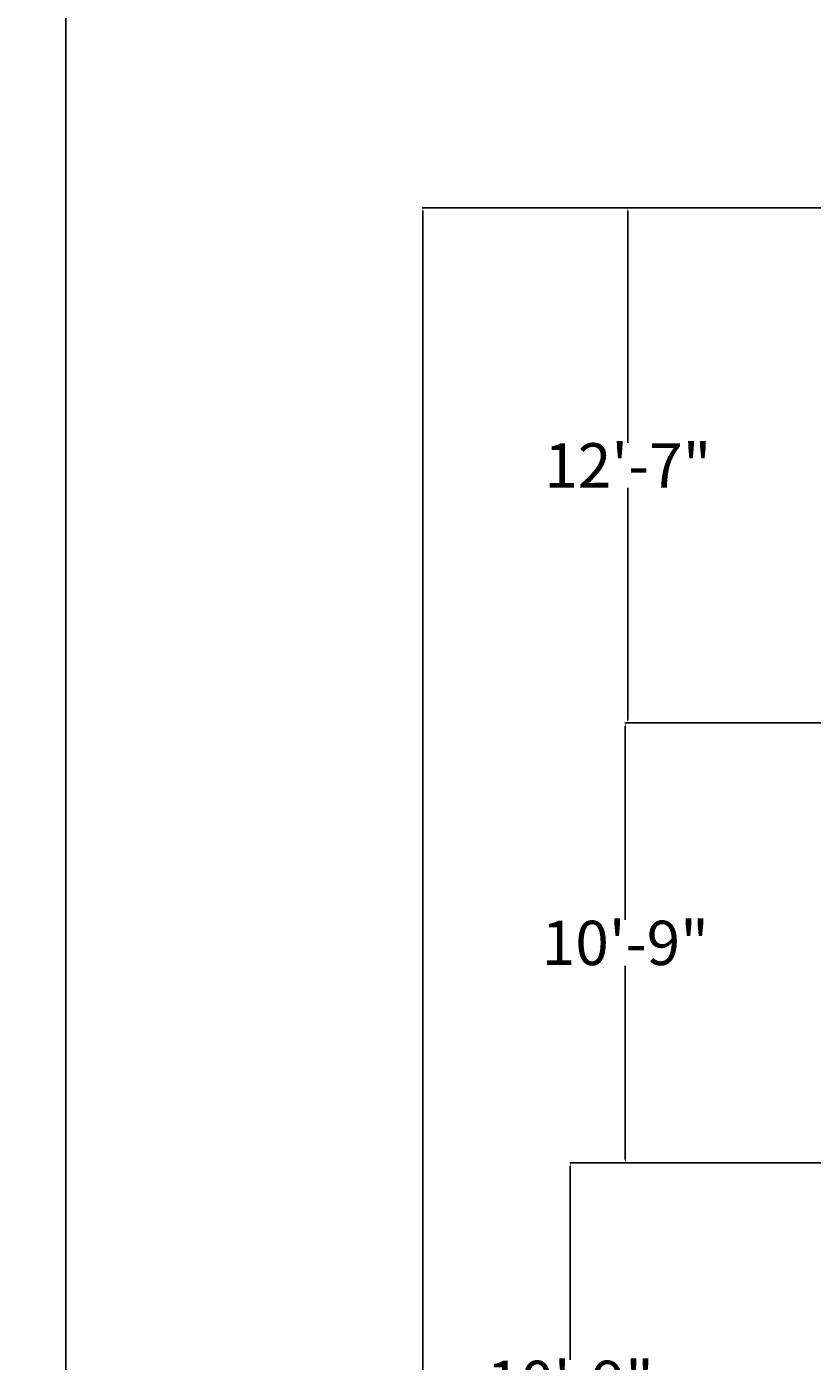
# Model space of a CAD drawing. Units: inches. Extents: x -364 to 705, y -52 to 1250.
# Tile 20 of 34: x -364 to -134, y 648 to 1039. Entities that reach past the tile are written whole.
import ezdxf

# ---------------------------------------------------------------- set-up
doc = ezdxf.new("R2010")
doc.units = ezdxf.units.IN
doc.header["$MEASUREMENT"] = 0
doc.layers.add('A-ANNO-DIMS', color=4, linetype='Continuous', lineweight=18)
doc.styles.get("Standard").update_dxf_attribs({"font": 'arial.ttf'})
doc.dimstyles.get("Standard").update_dxf_attribs({"dimtxt": 1, "dimasz": 1, "dimexe": 0.18, "dimexo": 0.0625, "dimgap": 0.09, "dimtad": 0, "dimtih": 1, "dimtoh": 1, "dimdec": 0, "dimzin": 0, "dimdsep": 46, "dimlunit": 3, "dimtxsty": 'Standard', "dimcen": 0.09, "dimadec": 0, "dimazin": 0, "dimtfac": 1, "dimtdec": 0, "dimtofl": 0, "dimtmove": 0, "dimatfit": 3, "dimfxl": 1, "dimtolj": 1, "dimtzin": 0, "dimarcsym": 0})

# ---------------------------------------------------------------- blocks, each defined once
blk = doc.blocks.new('*D18')
at = {"layer": 'A-ANNO-DIMS', "color": 0, "lineweight": -2, "transparency": 16777216}
for p, q in [((-254.46, 1079.11), (-353.05, 1079.11)), ((-352.87, 1078.11), (-352.87, 551.84)), ((-352.87, 12.11), (-352.87, 538.39)), ((-254.46, 11.11), (-353.05, 11.11))]:
    blk.add_line(p, q, dxfattribs=at)
at = {"layer": 'A-ANNO-DIMS', "color": 0, "transparency": 16777216}
for points in [[(-353.04, 1078.11), (-352.7, 1078.11), (-352.87, 1079.11)], [(-353.04, 12.11), (-352.7, 12.11), (-352.87, 11.11)]]:
    blk.add_solid(points, dxfattribs=at)
at = {"layer": 'Defpoints', "color": 0, "transparency": 16777216}
for p in [(-254.4, 1079.11), (-352.87, 11.11), (-254.4, 11.11)]:
    blk.add_point(p, dxfattribs=at)
at = {"layer": 'A-ANNO-DIMS', "color": 0, "transparency": 16777216, "insert": (-352.87, 545.11), "char_height": 1, "width": 1.6985, "attachment_point": 5}
blk.add_mtext("\\A1;{\\H13x;89'}", dxfattribs=at)
blk = doc.blocks.new('*D19')
at = {"layer": 'A-ANNO-DIMS', "color": 0, "lineweight": -2, "transparency": 16777216}
for p, q in [((28.52, 986.11), (-248.33, 986.11)), ((-248.15, 985.11), (-248.15, 574.22)), ((-248.15, 149.87), (-248.15, 560.77)), ((28.52, 148.87), (-248.33, 148.87))]:
    blk.add_line(p, q, dxfattribs=at)
at = {"layer": 'A-ANNO-DIMS', "color": 0, "transparency": 16777216}
for points in [[(-248.32, 985.11), (-247.99, 985.11), (-248.15, 986.11)], [(-248.32, 149.87), (-247.99, 149.87), (-248.15, 148.87)]]:
    blk.add_solid(points, dxfattribs=at)
at = {"layer": 'Defpoints', "color": 0, "transparency": 16777216}
for p in [(28.58, 986.11), (-248.15, 148.87), (28.58, 148.87)]:
    blk.add_point(p, dxfattribs=at)
at = {"layer": 'A-ANNO-DIMS', "color": 0, "transparency": 16777216, "insert": (-248.15, 567.49), "char_height": 1, "attachment_point": 5}
blk.add_mtext('\\A1;{\\H13x;69\'-9"}', dxfattribs=at)
blk = doc.blocks.new('*D20')
at = {"layer": 'A-ANNO-DIMS', "color": 0, "lineweight": -2, "transparency": 16777216}
for p, q in [((28.52, 986.11), (-188.21, 986.11)), ((-188.03, 985.11), (-188.03, 917.23)), ((-188.03, 836.11), (-188.03, 904)), ((37.52, 835.11), (-188.21, 835.11))]:
    blk.add_line(p, q, dxfattribs=at)
at = {"layer": 'A-ANNO-DIMS', "color": 0, "transparency": 16777216}
for points in [[(-188.19, 985.11), (-187.86, 985.11), (-188.03, 986.11)], [(-188.19, 836.11), (-187.86, 836.11), (-188.03, 835.11)]]:
    blk.add_solid(points, dxfattribs=at)
at = {"layer": 'Defpoints', "color": 0, "transparency": 16777216}
for p in [(28.58, 986.11), (-188.03, 835.11), (37.58, 835.11)]:
    blk.add_point(p, dxfattribs=at)
at = {"layer": 'A-ANNO-DIMS', "color": 0, "transparency": 16777216, "insert": (-188.03, 910.61), "char_height": 1, "attachment_point": 5}
blk.add_mtext('\\A1;{\\H13x;12\'-7"}', dxfattribs=at)
blk = doc.blocks.new('*D21')
at = {"layer": 'A-ANNO-DIMS', "color": 0, "lineweight": -2, "transparency": 16777216}
for p, q in [((37.52, 835.11), (-188.94, 835.11)), ((-188.76, 834.11), (-188.76, 777.34)), ((-188.76, 707.11), (-188.76, 763.89)), ((37.52, 706.11), (-188.94, 706.11))]:
    blk.add_line(p, q, dxfattribs=at)
at = {"layer": 'A-ANNO-DIMS', "color": 0, "transparency": 16777216}
for points in [[(-188.93, 834.11), (-188.59, 834.11), (-188.76, 835.11)], [(-188.93, 707.11), (-188.59, 707.11), (-188.76, 706.11)]]:
    blk.add_solid(points, dxfattribs=at)
at = {"layer": 'Defpoints', "color": 0, "transparency": 16777216}
for p in [(37.58, 835.11), (-188.76, 706.11), (37.58, 706.11)]:
    blk.add_point(p, dxfattribs=at)
at = {"layer": 'A-ANNO-DIMS', "color": 0, "transparency": 16777216, "insert": (-188.76, 770.61), "char_height": 1, "attachment_point": 5}
blk.add_mtext('\\A1;{\\H13x;10\'-9"}', dxfattribs=at)
blk = doc.blocks.new('*D31')
at = {"layer": 'A-ANNO-DIMS', "color": 0, "lineweight": -2, "transparency": 16777216}
for p, q in [((37.52, 706.11), (-205.07, 706.11)), ((-204.89, 705.11), (-204.89, 648.34)), ((-204.89, 578.11), (-204.89, 634.89)), ((37.52, 577.11), (-205.07, 577.11))]:
    blk.add_line(p, q, dxfattribs=at)
at = {"layer": 'A-ANNO-DIMS', "color": 0, "transparency": 16777216}
for points in [[(-205.06, 705.11), (-204.73, 705.11), (-204.89, 706.11)], [(-205.06, 578.11), (-204.73, 578.11), (-204.89, 577.11)]]:
    blk.add_solid(points, dxfattribs=at)
at = {"layer": 'Defpoints', "color": 0, "transparency": 16777216}
for p in [(37.58, 706.11), (-204.89, 577.11), (37.58, 577.11)]:
    blk.add_point(p, dxfattribs=at)
at = {"layer": 'A-ANNO-DIMS', "color": 0, "transparency": 16777216, "insert": (-204.89, 641.61), "char_height": 1, "attachment_point": 5}
blk.add_mtext('\\A1;{\\H13x;10\'-9"}', dxfattribs=at)

msp = doc.modelspace()

# ---------------------------------------------------------------- dimensions: what is measured, and where the dimension line sits
at = {"layer": 'A-ANNO-DIMS'}
for base, p1, p2, picture, middle in [((-352.87, 11.11), (-254.4, 1079.11), (-254.4, 11.11), '*D18', (-352.87, 545.11)), ((-248.15, 148.87), (28.58, 986.11), (28.58, 148.87), '*D19', (-248.15, 567.49)), ((-188.76, 706.11), (37.58, 835.11), (37.58, 706.11), '*D21', (-188.76, 770.61)), ((-204.89, 577.11), (37.58, 706.11), (37.58, 577.11), '*D31', (-204.89, 641.61))]:
    dim = msp.add_linear_dim(base=base, p1=p1, p2=p2, angle=90, text='{\\H13x;<>}', dimstyle='Standard', override={"dimclrd": 0, "dimclre": 0, "dimclrt": 0}, dxfattribs=at)
    dim.commit()
    dim.dimension.update_dxf_attribs({"geometry": picture, "text_midpoint": middle})
dim = msp.add_linear_dim(base=(-188.03, 835.11), p1=(28.58, 986.11), p2=(37.58, 835.11), angle=90, text='{\\H13x;<>}', dimstyle='Standard', override={"dimclrd": 0, "dimclre": 0, "dimclrt": 0}, dxfattribs=at)
dim.commit()
dim.dimension.update_dxf_attribs({"geometry": '*D20', "text_midpoint": (-188.03, 910.61), "dimtype": 160})

doc.saveas('drawing.dxf')
